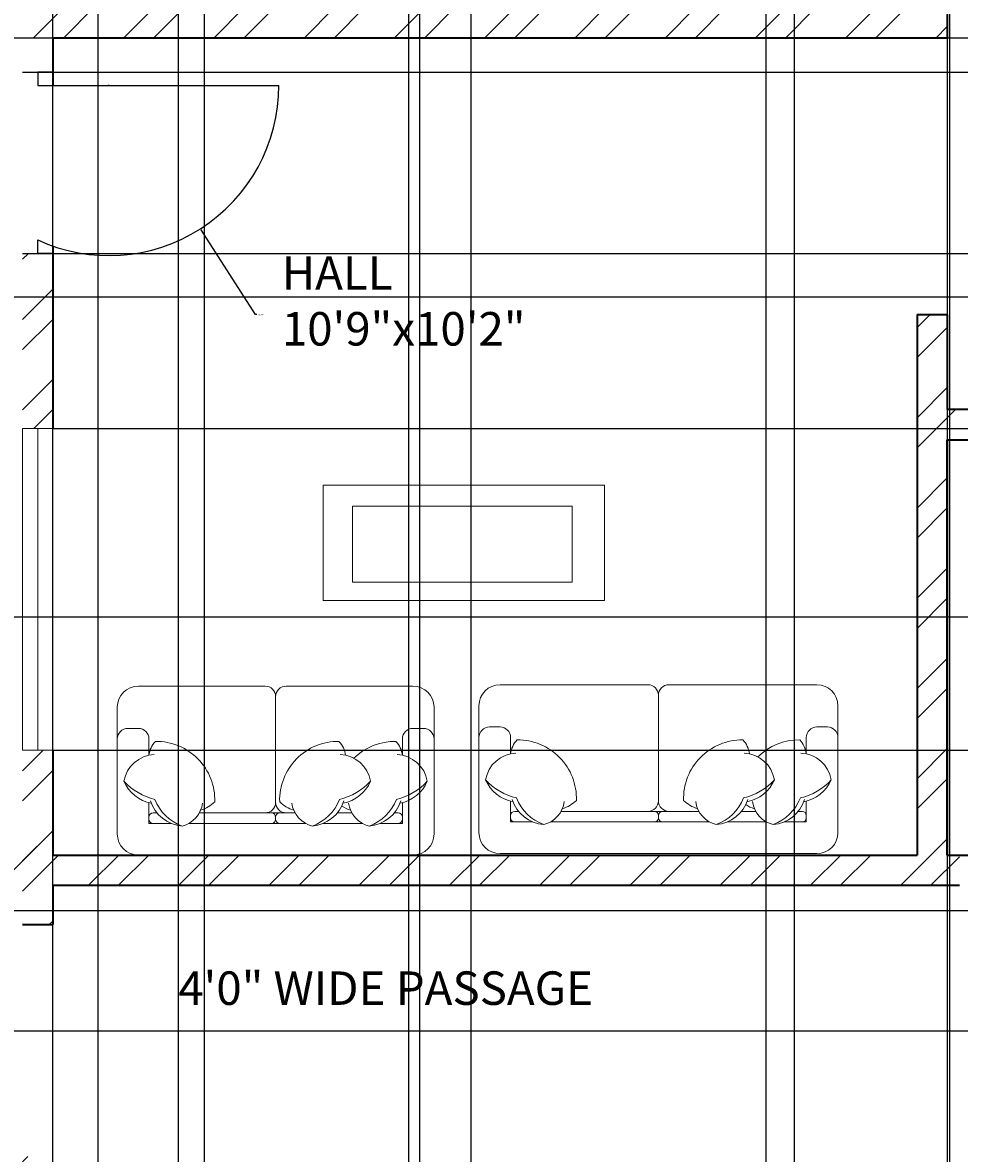
# Model space of a CAD drawing. Units: inches. Extents: x 2529 to 3014, y 1203 to 2262.
# Tile 7 of 13: x 2733 to 2873, y 1746 to 1915. Entities that reach past the tile are written whole.
import ezdxf

# ---------------------------------------------------------------- set-up
doc = ezdxf.new("R2010")
doc.units = ezdxf.units.IN
for name, color, linetype, lineweight in [('A-ANNO-DIMS', 2, 'Continuous', 18), ('A-AREA-IDEN', 7, 'Continuous', 18), ('A-DOOR', 21, 'Continuous', 25), ('A-FURN', 8, 'Continuous', 18), ('A-GLAZ', 191, 'Continuous', 18), ('A-WALL', 7, 'Continuous', 35), ('A-WALL-PATT', 143, 'Continuous', 13)]:
    doc.layers.add(name, color=color, linetype=linetype, lineweight=lineweight)
doc.styles.get("Standard").update_dxf_attribs({"font": 'arial.ttf'})
doc.dimstyles.get("Standard").update_dxf_attribs({"dimtxt": 0.18, "dimasz": 0.18, "dimexe": 0.18, "dimexo": 0.0625, "dimgap": 0.09, "dimtad": 0, "dimtih": 1, "dimtoh": 1, "dimdec": 4, "dimzin": 0, "dimdsep": 46, "dimtxsty": 'Standard', "dimcen": 0.09, "dimadec": 0, "dimazin": 0, "dimtfac": 1, "dimtdec": 4, "dimtofl": 0, "dimtmove": 0, "dimatfit": 3, "dimfxl": 1, "dimtolj": 1, "dimtzin": 0, "dimarcsym": 0})

# ---------------------------------------------------------------- blocks, each defined once
blk = doc.blocks.new('TABLE-COFFEE')
for points in [[(0, 41.99), (17.26, 41.99), (17.26, 0), (0, 0)], [(2.75, 37.58), (14.12, 37.58), (14.12, 4.82), (2.75, 4.82)]]:
    blk.add_lwpolyline(points, close=True)
blk = doc.blocks.new('*D36')
at = {"layer": 'A-ANNO-DIMS', "color": 0, "lineweight": -2, "transparency": 16777216}
for p, q in [((2737.56, 1582.57), (2737.56, 2243.11)), ((2756.33, 1582.57), (2756.33, 2243.11)), ((2737.74, 2242.93), (2746.49, 2242.93)), ((2756.15, 2242.93), (2747.4, 2242.93))]:
    blk.add_line(p, q, dxfattribs=at)
at = {"layer": 'A-ANNO-DIMS', "color": 0, "transparency": 16777216}
for points in [[(2737.74, 2242.96), (2737.74, 2242.9), (2737.56, 2242.93)], [(2756.15, 2242.96), (2756.15, 2242.9), (2756.33, 2242.93)]]:
    blk.add_solid(points, dxfattribs=at)
at = {"layer": 'Defpoints', "color": 0, "transparency": 16777216}
for p in [(2756.33, 2242.93), (2737.56, 1582.5), (2756.33, 1582.5)]:
    blk.add_point(p, dxfattribs=at)
at = {"layer": 'A-ANNO-DIMS', "color": 0, "transparency": 16777216, "insert": (2746.94, 2242.93), "char_height": 0.18, "attachment_point": 5}
blk.add_mtext('\\A1;18.778', dxfattribs=at)
blk = doc.blocks.new('*D37')
at = {"layer": 'A-ANNO-DIMS', "color": 0, "lineweight": -2, "transparency": 16777216}
for p, q in [((2756.33, 1582.57), (2756.33, 2243.11)), ((2792.33, 1582.57), (2792.33, 2243.11)), ((2756.51, 2242.93), (2774.11, 2242.93)), ((2792.15, 2242.93), (2774.55, 2242.93))]:
    blk.add_line(p, q, dxfattribs=at)
at = {"layer": 'A-ANNO-DIMS', "color": 0, "transparency": 16777216}
for points in [[(2756.51, 2242.96), (2756.51, 2242.9), (2756.33, 2242.93)], [(2792.15, 2242.96), (2792.15, 2242.9), (2792.33, 2242.93)]]:
    blk.add_solid(points, dxfattribs=at)
at = {"layer": 'Defpoints', "color": 0, "transparency": 16777216}
for p in [(2792.33, 2242.93), (2756.33, 1582.5), (2792.33, 1582.5)]:
    blk.add_point(p, dxfattribs=at)
at = {"layer": 'A-ANNO-DIMS', "color": 0, "transparency": 16777216, "insert": (2774.33, 2242.93), "char_height": 0.18, "attachment_point": 5}
blk.add_mtext('\\A1;36', dxfattribs=at)
blk = doc.blocks.new('*D38')
at = {"layer": 'A-ANNO-DIMS', "color": 0, "lineweight": -2, "transparency": 16777216}
for p, q in [((2844.06, 1582.57), (2844.06, 2243.11)), ((2871.44, 1582.57), (2871.44, 2243.11)), ((2844.24, 2242.93), (2857.35, 2242.93)), ((2871.26, 2242.93), (2858.14, 2242.93))]:
    blk.add_line(p, q, dxfattribs=at)
at = {"layer": 'A-ANNO-DIMS', "color": 0, "transparency": 16777216}
for points in [[(2844.24, 2242.96), (2844.24, 2242.9), (2844.06, 2242.93)], [(2871.26, 2242.96), (2871.26, 2242.9), (2871.44, 2242.93)]]:
    blk.add_solid(points, dxfattribs=at)
at = {"layer": 'Defpoints', "color": 0, "transparency": 16777216}
for p in [(2871.44, 2242.93), (2844.06, 1582.5), (2871.44, 1582.5)]:
    blk.add_point(p, dxfattribs=at)
at = {"layer": 'A-ANNO-DIMS', "color": 0, "transparency": 16777216, "insert": (2857.75, 2242.93), "char_height": 0.18, "attachment_point": 5}
blk.add_mtext('\\A1;27.39', dxfattribs=at)
blk = doc.blocks.new('*D39')
at = {"layer": 'A-ANNO-DIMS', "color": 0, "lineweight": -2, "transparency": 16777216}
for p, q in [((2848.27, 1734.07), (2848.27, 2243.11)), ((2881.26, 1734.07), (2881.26, 2243.11)), ((2848.45, 2242.93), (2864.3, 2242.93)), ((2881.08, 2242.93), (2865.23, 2242.93))]:
    blk.add_line(p, q, dxfattribs=at)
at = {"layer": 'A-ANNO-DIMS', "color": 0, "transparency": 16777216}
for points in [[(2848.45, 2242.96), (2848.45, 2242.9), (2848.27, 2242.93)], [(2881.08, 2242.96), (2881.08, 2242.9), (2881.26, 2242.93)]]:
    blk.add_solid(points, dxfattribs=at)
at = {"layer": 'Defpoints', "color": 0, "transparency": 16777216}
for p in [(2881.26, 2242.93), (2848.27, 1734), (2881.26, 1734)]:
    blk.add_point(p, dxfattribs=at)
at = {"layer": 'A-ANNO-DIMS', "color": 0, "transparency": 16777216, "insert": (2864.76, 2242.93), "char_height": 0.18, "attachment_point": 5}
blk.add_mtext('\\A1;32.994', dxfattribs=at)
blk = doc.blocks.new('*D40')
at = {"layer": 'A-ANNO-DIMS', "color": 0, "lineweight": -2, "transparency": 16777216}
for p, q in [((2744.32, 1738.57), (2744.32, 2243.11)), ((2800.02, 1738.57), (2800.02, 2243.11)), ((2744.5, 2242.93), (2771.84, 2242.93)), ((2799.84, 2242.93), (2772.49, 2242.93))]:
    blk.add_line(p, q, dxfattribs=at)
at = {"layer": 'A-ANNO-DIMS', "color": 0, "transparency": 16777216}
for points in [[(2744.5, 2242.96), (2744.5, 2242.9), (2744.32, 2242.93)], [(2799.84, 2242.96), (2799.84, 2242.9), (2800.02, 2242.93)]]:
    blk.add_solid(points, dxfattribs=at)
at = {"layer": 'Defpoints', "color": 0, "transparency": 16777216}
for p in [(2800.02, 2242.93), (2744.32, 1738.5), (2800.02, 1738.5)]:
    blk.add_point(p, dxfattribs=at)
at = {"layer": 'A-ANNO-DIMS', "color": 0, "transparency": 16777216, "insert": (2772.17, 2242.93), "char_height": 0.18, "attachment_point": 5}
blk.add_mtext('\\A1;55.7', dxfattribs=at)
blk = doc.blocks.new('*D57')
at = {"layer": 'A-ANNO-DIMS', "color": 0, "lineweight": -2, "transparency": 16777216}
for p, q in [((2871.06, 2198.44), (2871.06, 1483.77)), ((2893.92, 2198.44), (2893.92, 1483.77)), ((2871.24, 1483.95), (2882.02, 1483.95)), ((2893.74, 1483.95), (2882.95, 1483.95))]:
    blk.add_line(p, q, dxfattribs=at)
at = {"layer": 'A-ANNO-DIMS', "color": 0, "transparency": 16777216}
for points in [[(2871.24, 1483.98), (2871.24, 1483.92), (2871.06, 1483.95)], [(2893.74, 1483.98), (2893.74, 1483.92), (2893.92, 1483.95)]]:
    blk.add_solid(points, dxfattribs=at)
at = {"layer": 'Defpoints', "color": 0, "transparency": 16777216}
for p in [(2871.06, 2198.5), (2893.92, 2198.5), (2893.92, 1483.95)]:
    blk.add_point(p, dxfattribs=at)
at = {"layer": 'A-ANNO-DIMS', "color": 0, "transparency": 16777216, "insert": (2882.49, 1483.95), "char_height": 0.18, "attachment_point": 5}
blk.add_mtext('\\A1;22.866', dxfattribs=at)
blk = doc.blocks.new('*D62')
at = {"layer": 'A-ANNO-DIMS', "color": 0, "lineweight": -2, "transparency": 16777216}
for p, q in [((2904.99, 1782.69), (2541.45, 1782.69)), ((2541.63, 1782.51), (2541.63, 1773.88)), ((2541.63, 1764.89), (2541.63, 1773.52)), ((2904.99, 1764.71), (2541.45, 1764.71))]:
    blk.add_line(p, q, dxfattribs=at)
at = {"layer": 'A-ANNO-DIMS', "color": 0, "transparency": 16777216}
for points in [[(2541.6, 1782.51), (2541.66, 1782.51), (2541.63, 1782.69)], [(2541.6, 1764.89), (2541.66, 1764.89), (2541.63, 1764.71)]]:
    blk.add_solid(points, dxfattribs=at)
at = {"layer": 'Defpoints', "color": 0, "transparency": 16777216}
for p in [(2905.06, 1782.69), (2541.63, 1764.71), (2905.06, 1764.71)]:
    blk.add_point(p, dxfattribs=at)
at = {"layer": 'A-ANNO-DIMS', "color": 0, "transparency": 16777216, "insert": (2541.63, 1773.7), "char_height": 0.18, "attachment_point": 5}
blk.add_mtext('\\A1;17.983', dxfattribs=at)
blk = doc.blocks.new('*D63')
at = {"layer": 'A-ANNO-DIMS', "color": 0, "lineweight": -2, "transparency": 16777216}
for p, q in [((2737.62, 1907.87), (3007.66, 1907.87)), ((3007.48, 1907.69), (3007.48, 1894.52)), ((3007.48, 1880.99), (3007.48, 1894.16)), ((2737.62, 1880.81), (3007.66, 1880.81))]:
    blk.add_line(p, q, dxfattribs=at)
at = {"layer": 'A-ANNO-DIMS', "color": 0, "transparency": 16777216}
for points in [[(3007.45, 1907.69), (3007.51, 1907.69), (3007.48, 1907.87)], [(3007.45, 1880.99), (3007.51, 1880.99), (3007.48, 1880.81)]]:
    blk.add_solid(points, dxfattribs=at)
at = {"layer": 'Defpoints', "color": 0, "transparency": 16777216}
for p in [(2737.56, 1907.87), (3007.48, 1907.87), (2737.56, 1880.81)]:
    blk.add_point(p, dxfattribs=at)
at = {"layer": 'A-ANNO-DIMS', "color": 0, "transparency": 16777216, "insert": (3007.48, 1894.34), "char_height": 0.18, "attachment_point": 5}
blk.add_mtext('\\A1;27.057', dxfattribs=at)
blk = doc.blocks.new('*D67')
at = {"layer": 'A-ANNO-DIMS', "color": 0, "lineweight": -2, "transparency": 16777216}
for p, q in [((2678.12, 1913), (3007.66, 1913)), ((3007.48, 1912.82), (3007.48, 1893.83)), ((3007.48, 1874.48), (3007.48, 1893.47)), ((2678.12, 1874.3), (3007.66, 1874.3))]:
    blk.add_line(p, q, dxfattribs=at)
at = {"layer": 'A-ANNO-DIMS', "color": 0, "transparency": 16777216}
for points in [[(3007.45, 1912.82), (3007.51, 1912.82), (3007.48, 1913)], [(3007.45, 1874.48), (3007.51, 1874.48), (3007.48, 1874.3)]]:
    blk.add_solid(points, dxfattribs=at)
at = {"layer": 'Defpoints', "color": 0, "transparency": 16777216}
for p in [(2678.06, 1913), (3007.48, 1913), (2678.06, 1874.3)]:
    blk.add_point(p, dxfattribs=at)
at = {"layer": 'A-ANNO-DIMS', "color": 0, "transparency": 16777216, "insert": (3007.48, 1893.65), "char_height": 0.18, "attachment_point": 5}
blk.add_mtext('\\A1;38.7', dxfattribs=at)
blk = doc.blocks.new('*D68')
at = {"layer": 'A-ANNO-DIMS', "color": 0, "lineweight": -2, "transparency": 16777216}
for p, q in [((2622.12, 1874.3), (3007.66, 1874.3)), ((3007.48, 1874.12), (3007.48, 1850.62)), ((3007.48, 1826.75), (3007.48, 1850.25)), ((2622.12, 1826.57), (3007.66, 1826.57))]:
    blk.add_line(p, q, dxfattribs=at)
at = {"layer": 'A-ANNO-DIMS', "color": 0, "transparency": 16777216}
for points in [[(3007.45, 1874.12), (3007.51, 1874.12), (3007.48, 1874.3)], [(3007.45, 1826.75), (3007.51, 1826.75), (3007.48, 1826.57)]]:
    blk.add_solid(points, dxfattribs=at)
at = {"layer": 'Defpoints', "color": 0, "transparency": 16777216}
for p in [(2622.06, 1874.3), (3007.48, 1874.3), (2622.06, 1826.57)]:
    blk.add_point(p, dxfattribs=at)
at = {"layer": 'A-ANNO-DIMS', "color": 0, "transparency": 16777216, "insert": (3007.48, 1850.43), "char_height": 0.18, "attachment_point": 5}
blk.add_mtext('\\A1;47.735', dxfattribs=at)
blk = doc.blocks.new('*D69')
at = {"layer": 'A-ANNO-DIMS', "color": 0, "lineweight": -2, "transparency": 16777216}
for p, q in [((2737.62, 1854.67), (3007.66, 1854.67)), ((3007.48, 1854.49), (3007.48, 1830.85)), ((3007.48, 1806.85), (3007.48, 1830.49)), ((2737.62, 1806.67), (3007.66, 1806.67))]:
    blk.add_line(p, q, dxfattribs=at)
at = {"layer": 'A-ANNO-DIMS', "color": 0, "transparency": 16777216}
for points in [[(3007.45, 1854.49), (3007.51, 1854.49), (3007.48, 1854.67)], [(3007.45, 1806.85), (3007.51, 1806.85), (3007.48, 1806.67)]]:
    blk.add_solid(points, dxfattribs=at)
at = {"layer": 'Defpoints', "color": 0, "transparency": 16777216}
for p in [(2737.56, 1854.67), (3007.48, 1854.67), (2737.56, 1806.67)]:
    blk.add_point(p, dxfattribs=at)
at = {"layer": 'A-ANNO-DIMS', "color": 0, "transparency": 16777216, "insert": (3007.48, 1830.67), "char_height": 0.18, "attachment_point": 5}
blk.add_mtext('\\A1;48', dxfattribs=at)
blk = doc.blocks.new('*D70')
at = {"layer": 'A-ANNO-DIMS', "color": 0, "lineweight": -2, "transparency": 16777216}
for p, q in [((2737.62, 1880.81), (3007.66, 1880.81)), ((3007.48, 1880.63), (3007.48, 1867.92)), ((3007.48, 1854.85), (3007.48, 1867.56)), ((2737.62, 1854.67), (3007.66, 1854.67))]:
    blk.add_line(p, q, dxfattribs=at)
at = {"layer": 'A-ANNO-DIMS', "color": 0, "transparency": 16777216}
for points in [[(3007.45, 1880.63), (3007.51, 1880.63), (3007.48, 1880.81)], [(3007.45, 1854.85), (3007.51, 1854.85), (3007.48, 1854.67)]]:
    blk.add_solid(points, dxfattribs=at)
at = {"layer": 'Defpoints', "color": 0, "transparency": 16777216}
for p in [(2737.56, 1880.81), (3007.48, 1880.81), (2737.56, 1854.67)]:
    blk.add_point(p, dxfattribs=at)
at = {"layer": 'A-ANNO-DIMS', "color": 0, "transparency": 16777216, "insert": (3007.48, 1867.74), "char_height": 0.18, "attachment_point": 5}
blk.add_mtext('\\A1;26.14', dxfattribs=at)
blk = doc.blocks.new('*D78')
at = {"layer": 'A-ANNO-DIMS', "color": 0, "lineweight": -2, "transparency": 16777216}
for p, q in [((2760.22, 1599.16), (2760.22, 2243.11)), ((2790.72, 1599.16), (2790.72, 2243.11)), ((2760.4, 2242.93), (2775.15, 2242.93)), ((2790.54, 2242.93), (2775.8, 2242.93))]:
    blk.add_line(p, q, dxfattribs=at)
at = {"layer": 'A-ANNO-DIMS', "color": 0, "transparency": 16777216}
for points in [[(2760.4, 2242.96), (2760.4, 2242.9), (2760.22, 2242.93)], [(2790.54, 2242.96), (2790.54, 2242.9), (2790.72, 2242.93)]]:
    blk.add_solid(points, dxfattribs=at)
at = {"layer": 'Defpoints', "color": 0, "transparency": 16777216}
for p in [(2790.72, 2242.93), (2760.22, 1599.1), (2790.72, 1599.1)]:
    blk.add_point(p, dxfattribs=at)
at = {"layer": 'A-ANNO-DIMS', "color": 0, "transparency": 16777216, "insert": (2775.47, 2242.93), "char_height": 0.18, "attachment_point": 5}
blk.add_mtext('\\A1;30.5', dxfattribs=at)
blk = doc.blocks.new('*D87')
at = {"layer": 'A-ANNO-DIMS', "color": 0, "lineweight": -2, "transparency": 16777216}
for p, q in [((2745.83, 1905.87), (2746.01, 1905.87)), ((2745.92, 1905.78), (2745.92, 1905.96)), ((2767.83, 1871.67), (2759.71, 1884.34)), ((2768.01, 1871.67), (2767.83, 1871.67))]:
    blk.add_line(p, q, dxfattribs=at)
at = {"layer": 'A-ANNO-DIMS', "color": 0, "transparency": 16777216}
blk.add_solid([(2759.73, 1884.36), (2759.68, 1884.33), (2759.61, 1884.49)], dxfattribs=at)
at = {"layer": 'Defpoints', "color": 0, "transparency": 16777216}
for p in [(2745.92, 1905.87), (2759.61, 1884.49)]:
    blk.add_point(p, dxfattribs=at)
at = {"layer": 'A-ANNO-DIMS', "color": 0, "transparency": 16777216, "insert": (2768.56, 1871.67), "char_height": 0.18, "attachment_point": 5}
blk.add_mtext('\\A1;R25.384', dxfattribs=at)

msp = doc.modelspace()

# ---------------------------------------------------------------- hatches: boundary and pattern name
at = {"layer": 'A-WALL-PATT'}
h = msp.add_hatch(dxfattribs=at)
h.set_pattern_fill('ANSI32', color=256)
h.paths.add_polyline_path([(2686.5554, 2106.5032), (2622.0554, 2106.5032), (2622.0554, 2109.2964), (2617.4223, 2109.2964), (2613.0554, 2109.2964), (2613.0554, 2106.5032), (2577.0554, 2106.5032), (2577.0554, 2092.6918), (2586.0554, 2092.6918), (2586.0554, 2102.0032), (2682.0554, 2102.0032), (2682.0554, 2099.9833), (2686.5554, 2099.9833), (2686.5554, 2102.0032)])
h.paths.add_polyline_path([(2695.2249, 2054.0032), (2686.5554, 2054.0032), (2686.5554, 2080.2316), (2684.3054, 2080.2316), (2682.0554, 2080.2316), (2682.0554, 2054.0032), (2586.0554, 2054.0032), (2586.0554, 2068.6918), (2577.0554, 2068.6918), (2577.0554, 2019.1229), (2586.0554, 2019.1229), (2586.0554, 2049.5032), (2695.2249, 2049.5032)])
h.paths.add_polyline_path([(2737.5554, 2049.5032), (2866.5554, 2049.5032), (2866.5554, 2045.0233), (2871.0554, 2045.0233), (2871.0554, 2049.5032), (2871.0554, 2172.5032), (2866.5554, 2172.5032), (2829.1265, 2172.5032), (2829.1265, 2168.0032), (2866.5554, 2168.0032), (2866.5554, 2054.0032), (2737.5554, 2054.0032), (2737.5554, 2056.4892), (2735.3054, 2056.4892), (2733.0554, 2056.4892), (2733.0554, 2049.5032), (2733.0554, 1917.5032), (2733.0554, 1913.0032), (2871.0554, 1913.0032), (2871.0554, 1924.9149), (2868.8054, 1924.9149), (2866.5554, 1924.9149), (2866.5554, 1917.5032), (2737.5554, 1917.5032)], flags=17)
h.paths.add_polyline_path([(2972.0554, 2207.5032), (2613.0554, 2207.5032), (2613.0554, 2205.5032), (2613.0554, 2188.9366), (2622.0554, 2188.9366), (2622.0554, 2198.5032), (2733.0554, 2198.5032), (2733.0554, 2084.8053), (2735.3054, 2084.8053), (2737.5554, 2084.8053), (2737.5554, 2168.0032), (2769.1265, 2168.0032), (2769.1265, 2170.2532), (2769.1265, 2172.5032), (2737.5554, 2172.5032), (2737.5554, 2198.5032), (2963.0554, 2198.5032), (2963.0554, 2093.5032), (2912.0586, 2093.5032), (2912.0586, 2089.0032), (2918.5554, 2089.0032), (2918.5554, 2031.8749), (2923.0554, 2031.8749), (2923.0554, 2089.0032), (2963.0554, 2089.0032), (2963.0554, 2010.0032), (2923.0554, 2010.0032), (2923.0554, 2011.9417), (2918.5554, 2011.9417), (2918.5554, 2003.1338), (2923.0554, 2003.1338), (2923.0554, 2005.5032), (2963.0554, 2005.5032), (2963.0554, 1917.5032), (2963.0554, 1691.0776), (2972.0554, 1691.0776), (2972.0554, 1917.5032)])
h.paths.add_polyline_path([(2963.0554, 1945.5032), (2923.0554, 1945.5032), (2923.0554, 1983.0571), (2920.8054, 1983.0571), (2918.5554, 1983.0571), (2918.5554, 1941.0032), (2963.0554, 1941.0032)], flags=17)
h.paths.add_polyline_path([(2930.3679, 1788.7532), (2930.3679, 1791.0032), (2894.8637, 1791.0032), (2894.8637, 1786.5032), (2900.5554, 1786.5032), (2900.5554, 1784.6931), (2905.0554, 1784.6931), (2905.0554, 1786.5032), (2930.3679, 1786.5032)], flags=17)
h.paths.add_polyline_path([(2963.0554, 1791.0032), (2954.3679, 1791.0032), (2954.3679, 1786.5032), (2963.0554, 1786.5032)], flags=17)
h.paths.add_polyline_path([(2871.0554, 1853.0032), (2919.0554, 1853.0032), (2919.0554, 1847.0972), (2923.5554, 1847.0972), (2923.5554, 1853.0032), (2923.5554, 1857.5032), (2871.0554, 1857.5032), (2871.0554, 1871.7024), (2866.5554, 1871.7024), (2866.5554, 1791.0032), (2737.5554, 1791.0032), (2737.5554, 1806.6712), (2735.3054, 1806.6712), (2733.0554, 1806.6712), (2733.0554, 1791.0032), (2733.0554, 1786.5032), (2733.0554, 1780.6235), (2737.5554, 1780.6235), (2737.5554, 1786.5032), (2872.8745, 1786.5032), (2872.8745, 1788.7532), (2872.8745, 1791.0032), (2871.0554, 1791.0032)], flags=17)
h.paths.add_polyline_path([(2844.0554, 1734.0032), (2848.2652, 1734.0032), (2848.2652, 1738.5032), (2800.0167, 1738.5032), (2800.0167, 1734.0032), (2839.5554, 1734.0032), (2839.5554, 1582.5032), (2792.3334, 1582.5032), (2792.3334, 1573.5032), (2871.4433, 1573.5032), (2871.4433, 1578.0032), (2871.4433, 1582.5032), (2844.0554, 1582.5032)])
h.paths.add_polyline_path([(2972.0554, 1631.0776), (2963.0554, 1631.0776), (2963.0554, 1582.5032), (2931.4433, 1582.5032), (2931.4433, 1573.5032), (2972.0554, 1573.5032)])
h.paths.add_polyline_path([(2756.3334, 1582.5032), (2737.5554, 1582.5032), (2737.5554, 1734.0032), (2744.3201, 1734.0032), (2744.3201, 1738.5032), (2737.5554, 1738.5032), (2737.5554, 1746.0094), (2733.0554, 1746.0094), (2733.0554, 1738.5032), (2733.0554, 1612.5032), (2728.2475, 1612.5032), (2728.2475, 1603.5032), (2733.0554, 1603.5032), (2733.0554, 1582.5032), (2733.0554, 1573.5032), (2756.3334, 1573.5032), (2756.3334, 1578.0032)])
h.paths.add_polyline_path([(2695.7662, 1612.5032), (2658.4771, 1612.5032), (2658.4771, 1603.5032), (2695.7662, 1603.5032), (2695.7662, 1608.0032)])
h.paths.add_polyline_path([(2586.0554, 1686.9483), (2577.0554, 1686.9483), (2577.0554, 1603.5032), (2598.4771, 1603.5032), (2598.4771, 1608.0032), (2598.4771, 1612.5032), (2586.0554, 1612.5032)])
h.paths.add_polyline_path([(2683.2727, 1791.0032), (2586.0554, 1791.0032), (2586.0554, 1815.6736), (2581.5554, 1815.6736), (2577.0554, 1815.6736), (2577.0554, 1746.9483), (2586.0554, 1746.9483), (2586.0554, 1786.5032), (2683.2727, 1786.5032)])
h.paths.add_polyline_path([(2586.0554, 1959.1229), (2577.0554, 1959.1229), (2577.0554, 1875.6736), (2586.0554, 1875.6736), (2586.0554, 1913.0032), (2683.2727, 1913.0032), (2683.2727, 1917.5032), (2586.0554, 1917.5032)])
h = msp.add_hatch(dxfattribs=at)
h.set_pattern_fill('ANSI32', color=256)
h.paths.add_polyline_path([(2737.5554, 1786.5032), (2872.8745, 1786.5032), (2872.8745, 1788.7532), (2872.8745, 1791.0032), (2871.0554, 1791.0032), (2871.0554, 1853.0032), (2919.0554, 1853.0032), (2919.0554, 1847.0972), (2923.5554, 1847.0972), (2923.5554, 1853.0032), (2923.5554, 1857.5032), (2871.0554, 1857.5032), (2871.0554, 1871.7024), (2866.5554, 1871.7024), (2866.5554, 1791.0032), (2737.5554, 1791.0032), (2737.5554, 1806.6712), (2735.3054, 1806.6712), (2733.0554, 1806.6712), (2733.0554, 1791.0032), (2730.085, 1791.0032), (2730.085, 1786.5032), (2733.0554, 1786.5032), (2733.0554, 1780.6235), (2737.5554, 1780.6235)])
h.paths.add_polyline_path([(2737.5554, 1880.8133), (2735.3054, 1880.8133), (2733.0554, 1880.8133), (2733.0554, 1854.6712), (2737.5554, 1854.6712)])
h.paths.add_polyline_path([(2695.1228, 1915.2532), (2695.1228, 1917.5032), (2586.0554, 1917.5032), (2586.0554, 1959.1229), (2577.0554, 1959.1229), (2577.0554, 1875.6736), (2586.0554, 1875.6736), (2586.0554, 1913.0032), (2695.1228, 1913.0032)])
h = msp.add_hatch(dxfattribs=at)
h.set_pattern_fill('ANSI32', color=256)
h.paths.add_polyline_path([(2696.9325, 1791.0032), (2586.0554, 1791.0032), (2586.0554, 1815.6736), (2581.5554, 1815.6736), (2577.0554, 1815.6736), (2577.0554, 1746.9483), (2586.0554, 1746.9483), (2586.0554, 1786.5032), (2696.9325, 1786.5032)])
h.paths.add_polyline_path([(2872.8745, 1791.0032), (2871.0554, 1791.0032), (2871.0554, 1853.0032), (2919.0554, 1853.0032), (2919.0554, 1847.0972), (2923.5554, 1847.0972), (2923.5554, 1853.0032), (2923.5554, 1857.5032), (2871.0554, 1857.5032), (2871.0554, 1871.7024), (2866.5554, 1871.7024), (2866.5554, 1791.0032), (2737.5554, 1791.0032), (2737.5554, 1806.6712), (2735.3054, 1806.6712), (2733.0554, 1806.6712), (2733.0554, 1791.0032), (2730.085, 1791.0032), (2730.085, 1786.5032), (2733.0554, 1786.5032), (2733.0554, 1780.6235), (2737.5554, 1780.6235), (2737.5554, 1786.5032), (2872.8745, 1786.5032), (2872.8745, 1788.7532)])

# ---------------------------------------------------------------- linework, layer by layer
at = {"layer": 'A-DOOR'}
for p, q in [((2733.0554, 1907.8704), (2737.5554, 1907.8704)), ((2737.5554, 1907.8704), (2735.3054, 1907.8704)), ((2735.3054, 1907.8704), (2735.3054, 1905.8704)), ((2735.3054, 1905.8704), (2771.3054, 1905.8704)), ((2735.3054, 1880.8133), (2735.3054, 1882.8133)), ((2733.0554, 1880.8133), (2737.5554, 1880.8133)), ((2737.5554, 1880.8133), (2735.3054, 1880.8133))]:
    msp.add_line(p, q, dxfattribs=at)
msp.add_arc((2745.9216, 1905.8704), 25.3838, 245.277119, 0, dxfattribs=at)
at = {"layer": 'A-FURN', "ltscale": 0.03}
for points in [[(2769.2475, 1816.22, -0.41421356), (2770.8236, 1814.644, -0.41421356), (2772.3996, 1816.22), (2791.3122, 1816.22, -0.41421356), (2794.4643, 1813.0679), (2794.4643, 1794.1553, -0.41421356), (2791.3122, 1791.0032), (2750.3349, 1791.0032, -0.41421356), (2747.1828, 1794.1553), (2747.1828, 1813.0679, -0.41421356), (2750.3349, 1816.22), (2769.2475, 1816.22, -0.41421356), (2770.8236, 1814.644, -0.41421356), (2772.3996, 1816.22)], [(2826.3801, 1816.4317, -0.41421356), (2827.9561, 1814.8557, -0.41421356), (2829.5322, 1816.4317), (2851.5968, 1816.4317, -0.41421356), (2854.7489, 1813.2796), (2854.7489, 1794.3671, -0.41421356), (2851.5968, 1791.215), (2804.3154, 1791.215, -0.41421356), (2801.1633, 1794.3671), (2801.1633, 1813.2796, -0.41421356), (2804.3154, 1816.4317), (2826.3801, 1816.4317, -0.41421356), (2827.9561, 1814.8557, -0.41421356), (2829.5322, 1816.4317)]]:
    msp.add_lwpolyline(points, format="xyb", dxfattribs=at)
at = {"layer": 'A-FURN'}
for points in [[(2769.2475, 1797.3074, 0.41421356), (2770.8236, 1798.8835), (2770.8236, 1814.644, 0.41421356)], [(2772.3996, 1797.3074, -0.41421356), (2770.8236, 1798.8835), (2770.8236, 1814.644, -0.41421356)], [(2826.3801, 1797.5192, 0.41421356), (2827.9561, 1799.0952), (2827.9561, 1814.8557, 0.41421356)], [(2829.5322, 1797.5192, -0.41421356), (2827.9561, 1799.0952), (2827.9561, 1814.8557, -0.41421356)], [(2747.1828, 1808.3398, -0.41421356), (2748.7589, 1809.9158), (2750.3349, 1809.9158, -0.41421356), (2751.911, 1808.3398), (2751.911, 1805.8979)], [(2789.7361, 1805.8979), (2789.7361, 1808.3398, -0.41421356), (2791.3122, 1809.9158), (2792.8882, 1809.9158, -0.41421356), (2794.4643, 1808.3398)], [(2801.1633, 1808.5515, -0.41421356), (2802.7393, 1810.1275), (2804.3154, 1810.1275, -0.41421356), (2805.8914, 1808.5515), (2805.8914, 1806.1096)], [(2850.0208, 1806.1096), (2850.0208, 1808.5515, -0.41421356), (2851.5968, 1810.1275), (2853.1729, 1810.1275, -0.41421356), (2854.7489, 1808.5515)], [(2751.9075, 1805.8972, -0.16554063), (2752.8825, 1807.9796, -0.42598917), (2761.7339, 1798.9509, -0.12152332), (2759.6328, 1797.7065, 7.11546429)], [(2781.2495, 1805.8972, 0.16554063), (2780.2745, 1807.9796, 0.42598917), (2771.4231, 1798.9509, 0.12152332), (2773.5242, 1797.7065, -7.11546429)], [(2789.7396, 1805.8972, 0.16554063), (2788.7646, 1807.9796, 0.20023115), (2782.5082, 1805.4434, 0.12152332)], [(2805.888, 1806.1089, -0.16554063), (2806.863, 1808.1913, -0.42598917), (2815.7144, 1799.1627, -0.12152332), (2813.6133, 1797.9182, 7.11546429)], [(2841.5341, 1806.1089, 0.16554063), (2840.5591, 1808.1913, 0.42598917), (2831.7077, 1799.1627, 0.12152332), (2833.8089, 1797.9182, -7.11546429)], [(2850.0242, 1806.1089, 0.16554063), (2849.0492, 1808.1913, 0.20023115), (2842.7929, 1805.6552, 0.12152332)], [(2752.7019, 1805.9933, 0.35677236), (2748.1859, 1802.0207, 0.24954205), (2752.2778, 1798.7469, -9.61688035)], [(2780.4551, 1805.9933, -0.35677236), (2784.9711, 1802.0207, -0.24954205), (2780.8792, 1798.7469, 9.61688035)], [(2788.9452, 1805.9933, -0.35677236), (2793.4612, 1802.0207, -0.24954205), (2789.3693, 1798.7469, 9.61688035)], [(2806.6824, 1806.205, 0.35677236), (2802.1664, 1802.2324, 0.24954205), (2806.2583, 1798.9586, -9.61688035)], [(2840.7398, 1806.205, -0.35677236), (2845.2558, 1802.2324, -0.24954205), (2841.1639, 1798.9586, 9.61688035)], [(2849.2299, 1806.205, -0.35677236), (2853.7459, 1802.2324, -0.24954205), (2849.654, 1798.9586, 9.61688035)], [(2748.1859, 1802.0207, 0.14772988), (2752.7922, 1799.3121, 0.21334276), (2756.8566, 1795.3395, 0.17866181)], [(2784.9711, 1802.0207, -0.14772988), (2780.3648, 1799.3121, -0.21334276), (2776.3004, 1795.3395, -0.17866181)], [(2793.4612, 1802.0207, -0.14772988), (2788.8549, 1799.3121, -0.21334276), (2784.7905, 1795.3395, -0.17866181)], [(2802.1664, 1802.2324, 0.14772988), (2806.7727, 1799.5238, 0.21334276), (2810.8371, 1795.5512, 0.17866181)], [(2845.2558, 1802.2324, -0.14772988), (2840.6494, 1799.5238, -0.21334276), (2836.585, 1795.5512, -0.17866181)], [(2853.7459, 1802.2324, -0.14772988), (2849.1396, 1799.5238, -0.21334276), (2845.0751, 1795.5512, -0.17866181)], [(2806.1363, 1799.3079, 0.30666349), (2810.8371, 1795.5512, 0.30632997), (2813.908, 1798.9821, -0.87284716)], [(2841.2858, 1799.3079, -0.30666349), (2836.585, 1795.5512, -0.30632997), (2833.5141, 1798.9821, 0.87284716)], [(2849.7759, 1799.3079, -0.30666349), (2845.0751, 1795.5512, -0.30632997), (2842.0042, 1798.9821, 0.87284716)], [(2752.1559, 1799.0962, 0.30666349), (2756.8566, 1795.3395, 0.30632997), (2759.9275, 1798.7703, -0.87284716)], [(2769.2475, 1797.3074, 0.41421356), (2770.8236, 1798.8835)], [(2772.3996, 1797.3074, -0.41421356), (2770.8236, 1798.8835)], [(2781.0012, 1799.0962, -0.30666349), (2776.3004, 1795.3395, -0.30632997), (2773.2295, 1798.7703, 0.87284716)], [(2780.693, 1798.3226, 0.07186538), (2782.0143, 1797.7065, -7.11546429)], [(2789.4913, 1799.0962, -0.30666349), (2784.7905, 1795.3395, -0.30632997), (2781.7196, 1798.7703, 0.87284716)], [(2786.4206, 1795.7314), (2789.7361, 1795.7314), (2789.7361, 1798.8287, -0.41421356)], [(2807.0942, 1797.5192), (2806.5219, 1797.5192, 0.41421356), (2805.8914, 1796.8887), (2805.8914, 1796.5735, 0.41421356), (2806.5219, 1795.9431)], [(2811.829, 1795.9431), (2827.3257, 1795.9431, 0.41421356), (2827.9561, 1796.5735), (2827.9561, 1796.8887, 0.41421356), (2827.3257, 1797.5192), (2813.416, 1797.5192, 0.41421356)], [(2826.3801, 1797.5192, 0.41421356), (2827.9561, 1799.0952)], [(2829.5322, 1797.5192, -0.41421356), (2827.9561, 1799.0952)], [(2835.5931, 1795.9431), (2828.5865, 1795.9431, -0.41421356), (2827.9561, 1796.5735), (2827.9561, 1796.8887, -0.41421356), (2828.5865, 1797.5192), (2834.0062, 1797.5192, -0.41421356)], [(2840.328, 1797.5192), (2842.4963, 1797.5192, -0.41421356)], [(2840.9777, 1798.5344, 0.07186538), (2842.299, 1797.9182, -7.11546429)], [(2846.7052, 1795.9431), (2850.0208, 1795.9431), (2850.0208, 1799.0404, -0.41421356)], [(2848.8181, 1797.5192), (2849.3904, 1797.5192, -0.41421356), (2850.0208, 1796.8887), (2850.0208, 1796.5735, -0.41421356), (2849.3904, 1795.9431)], [(2753.1137, 1797.3074), (2752.5414, 1797.3074, 0.41421356), (2751.911, 1796.677), (2751.911, 1796.3618, 0.41421356), (2752.5414, 1795.7314)], [(2757.8485, 1795.7314), (2770.1931, 1795.7314, 0.41421356), (2770.8236, 1796.3618), (2770.8236, 1796.677, 0.41421356), (2770.1931, 1797.3074), (2759.4355, 1797.3074, 0.41421356)], [(2775.3085, 1795.7314), (2771.454, 1795.7314, -0.41421356), (2770.8236, 1796.3618), (2770.8236, 1796.677, -0.41421356), (2771.454, 1797.3074), (2773.7215, 1797.3074, -0.41421356)], [(2780.0433, 1797.3074), (2782.2116, 1797.3074, -0.41421356)], [(2788.5334, 1797.3074), (2789.1057, 1797.3074, -0.41421356), (2789.7361, 1796.677), (2789.7361, 1796.3618, -0.41421356), (2789.1057, 1795.7314)], [(2806.5219, 1795.9431), (2809.207, 1795.9431, 0.41421356)], [(2844.0833, 1795.9431), (2838.2151, 1795.9431, -0.41421356)], [(2849.3904, 1795.9431), (2846.7052, 1795.9431, -0.41421356)], [(2752.5414, 1795.7314), (2755.2265, 1795.7314, 0.41421356)], [(2783.7986, 1795.7314), (2777.9305, 1795.7314, -0.41421356)], [(2789.1057, 1795.7314), (2786.4206, 1795.7314, -0.41421356)]]:
    msp.add_lwpolyline(points, format="xyb", dxfattribs=at)
for points in [[(2751.911, 1798.8287), (2751.911, 1795.7314), (2755.2265, 1795.7314)], [(2805.8914, 1799.0404), (2805.8914, 1795.9431), (2809.207, 1795.9431)], [(2811.829, 1795.9431), (2835.5931, 1795.9431)], [(2838.2151, 1795.9431), (2844.0833, 1795.9431)], [(2757.8485, 1795.7314), (2775.3085, 1795.7314)], [(2777.9305, 1795.7314), (2783.7986, 1795.7314)]]:
    msp.add_lwpolyline(points, dxfattribs=at)
for points in [[(2827.3257, 1795.9431), (2828.5865, 1795.9431, -0.41421356), (2827.9561, 1796.5735), (2827.9561, 1796.8887, -0.41421356), (2828.5865, 1797.5192), (2827.3257, 1797.5192, -0.41421356), (2827.9561, 1796.8887), (2827.9561, 1796.5735, -0.41421356)], [(2770.1931, 1795.7314), (2771.454, 1795.7314, -0.41421356), (2770.8236, 1796.3618), (2770.8236, 1796.677, -0.41421356), (2771.454, 1797.3074), (2770.1931, 1797.3074, -0.41421356), (2770.8236, 1796.677), (2770.8236, 1796.3618, -0.41421356)]]:
    msp.add_lwpolyline(points, format="xyb", close=True, dxfattribs=at)
at = {"layer": 'A-GLAZ'}
for p, q in [((2735.3054, 1854.6712), (2733.0554, 1854.6712)), ((2733.0554, 1854.6712), (2737.5554, 1854.6712)), ((2733.0554, 1854.6712), (2733.0554, 1806.6712)), ((2735.3054, 1806.6712), (2735.3054, 1854.6712)), ((2737.5554, 1854.6712), (2737.5554, 1806.6712)), ((2733.0554, 1806.6712), (2737.5554, 1806.6712)), ((2737.5554, 1806.6712), (2735.3054, 1806.6712))]:
    msp.add_line(p, q, dxfattribs=at)
at = {"layer": 'A-WALL'}
for p, q in [((2871.0554, 1924.9149), (2871.0554, 1913.0032)), ((2737.5554, 1913.0032), (2871.0554, 1913.0032)), ((2737.5554, 1913.0032), (2737.5554, 1905.8704)), ((2737.5554, 1881.905), (2737.5554, 1854.6712)), ((2866.5554, 1871.7024), (2866.5554, 1791.0032)), ((2866.5554, 1871.7024), (2871.0554, 1871.7024)), ((2871.0554, 1871.7024), (2871.0554, 1857.5032)), ((2923.5554, 1857.5032), (2871.0554, 1857.5032)), ((2871.0554, 1791.0032), (2871.0554, 1853.0032)), ((2871.0554, 1853.0032), (2919.0554, 1853.0032)), ((2871.0554, 1853.0032), (2871.0554, 1791.0032)), ((2737.5554, 1806.6712), (2737.5554, 1791.0032)), ((2737.5554, 1791.0032), (2866.5554, 1791.0032)), ((2871.0554, 1791.0032), (2874.8745, 1791.0032)), ((2737.5554, 1786.5032), (2737.5554, 1780.6235)), ((2737.5554, 1786.5032), (2872.8745, 1786.5032)), ((2733.0554, 1780.6235), (2737.5554, 1780.6235))]:
    msp.add_line(p, q, dxfattribs=at)

# ---------------------------------------------------------------- block references
at = {"layer": 'A-FURN', "rotation": 90.00000000000082}
msp.add_blockref('TABLE-COFFEE', (2819.8816, 1828.9782), dxfattribs=at)

# ---------------------------------------------------------------- texts
at = {"layer": 'A-AREA-IDEN', "char_height": 5, "attachment_point": 1}
for s, width, insert in [('HALL\\P10\'9"x10\'2"', 162.316117, (2771.7456, 1880.3856)), ('4\'0" WIDE PASSAGE', 108.755322, (2756.2875, 1773.6417))]:
    msp.add_mtext_dynamic_manual_height_columns(s, width=width, gutter_width=12.5, heights=[0], dxfattribs=dict(at, insert=insert))

# ---------------------------------------------------------------- dimensions: what is measured, and where the dimension line sits
at = {"layer": 'A-ANNO-DIMS'}
for base, p1, p2, override, picture, middle in [((2756.3334, 2242.9282), (2737.5554, 1582.5032), (2756.3334, 1582.5032), {"dimdec": 3, "dimlfac": 1, "dimrnd": 0, "dimzin": 0, "dimdsep": 46, "dimlunit": 2}, '*D36', (2746.9444, 2242.9282)), ((2800.0167, 2242.9282), (2744.3201, 1738.5032), (2800.0167, 1738.5032), {"dimdec": 1, "dimlfac": 1, "dimrnd": 0, "dimzin": 0, "dimdsep": 46, "dimlunit": 2}, '*D40', (2772.1684, 2242.9282)), ((2792.3334, 2242.9282), (2756.3334, 1582.5032), (2792.3334, 1582.5032), {"dimdec": 0, "dimlfac": 1, "dimrnd": 0, "dimzin": 0, "dimdsep": 46, "dimlunit": 2}, '*D37', (2774.3334, 2242.9282)), ((2790.721, 2242.9282), (2760.2227, 1599.0994), (2790.721, 1599.0994), {"dimdec": 1, "dimlfac": 1, "dimrnd": 0, "dimzin": 0, "dimdsep": 46, "dimlunit": 2}, '*D78', (2775.4718, 2242.9282)), ((2871.4433, 2242.9282), (2844.0554, 1582.5032), (2871.4433, 1582.5032), {"dimdec": 2, "dimlfac": 1, "dimrnd": 0, "dimzin": 0, "dimdsep": 46, "dimlunit": 2}, '*D38', (2857.7493, 2242.9282)), ((2881.259, 2242.9282), (2848.2652, 1734.0032), (2881.259, 1734.0032), {"dimdec": 3, "dimlfac": 1, "dimrnd": 0, "dimzin": 0, "dimdsep": 46, "dimlunit": 2}, '*D39', (2864.7621, 2242.9282)), ((2893.9216, 1483.9492), (2871.0554, 2198.5032), (2893.9216, 2198.5032), {"dimdec": 3, "dimlfac": 1, "dimrnd": 0, "dimzin": 0, "dimdsep": 46, "dimlunit": 2}, '*D57', (2882.4885, 1483.9492))]:
    dim = msp.add_linear_dim(base=base, p1=p1, p2=p2, dimstyle='Standard', override=override, dxfattribs=at)
    dim.commit()
    dim.dimension.update_dxf_attribs({"geometry": picture, "text_midpoint": middle})
for base, p1, p2, override, picture, middle in [((3007.4804, 1913.0032), (2678.0554, 1874.3024), (2678.0554, 1913.0032), {"dimdec": 1, "dimlfac": 1, "dimrnd": 0, "dimzin": 0, "dimdsep": 46, "dimlunit": 2}, '*D67', (3007.4804, 1893.6528)), ((3007.4804, 1907.8704), (2737.5554, 1880.8133), (2737.5554, 1907.8704), {"dimdec": 3, "dimlfac": 1, "dimrnd": 0, "dimzin": 0, "dimdsep": 46, "dimlunit": 2}, '*D63', (3007.4804, 1894.3419)), ((3007.4804, 1880.8133), (2737.5554, 1854.6712), (2737.5554, 1880.8133), {"dimdec": 2, "dimlfac": 1, "dimrnd": 0, "dimzin": 0, "dimdsep": 46, "dimlunit": 2}, '*D70', (3007.4804, 1867.7422)), ((3007.4804, 1874.3024), (2622.0554, 1826.5675), (2622.0554, 1874.3024), {"dimdec": 3, "dimlfac": 1, "dimrnd": 0, "dimzin": 0, "dimdsep": 46, "dimlunit": 2}, '*D68', (3007.4804, 1850.435)), ((3007.4804, 1854.6712), (2737.5554, 1806.6712), (2737.5554, 1854.6712), {"dimdec": 0, "dimlfac": 1, "dimrnd": 0, "dimzin": 0, "dimdsep": 46, "dimlunit": 2}, '*D69', (3007.4804, 1830.6712)), ((2541.6304, 1764.7097), (2905.0554, 1782.6931), (2905.0554, 1764.7097), {"dimdec": 3, "dimlfac": 1, "dimrnd": 0, "dimzin": 0, "dimdsep": 46, "dimlunit": 2}, '*D62', (2541.6304, 1773.7014))]:
    dim = msp.add_linear_dim(base=base, p1=p1, p2=p2, angle=90, dimstyle='Standard', override=override, dxfattribs=at)
    dim.commit()
    dim.dimension.update_dxf_attribs({"geometry": picture, "text_midpoint": middle})
dim = msp.add_radius_dim(center=(2745.9216, 1905.8704), mpoint=(2759.612, 1884.495), dimstyle='Standard', override={"dimdec": 3, "dimlfac": 1, "dimrnd": 0, "dimzin": 0, "dimdsep": 46, "dimlunit": 2}, dxfattribs=at)
dim.commit()
dim.dimension.update_dxf_attribs({"geometry": '*D87', "text_midpoint": (2768.5556, 1871.6698), "dimtype": 164})

doc.saveas('drawing.dxf')
